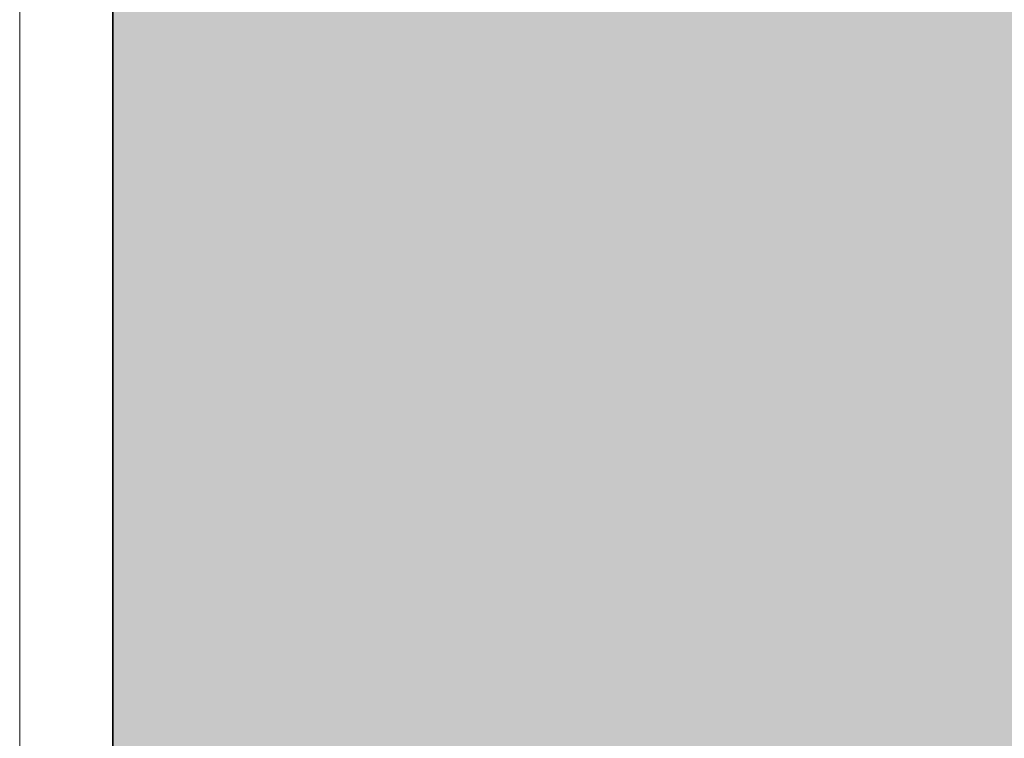
# Model space of a CAD drawing. Units: inches. Extents: x 2091 to 2899, y 967 to 2217.
# Tile 221 of 256: x 2203.1157 to 2203.4104, y 1152.4622 to 1152.6774. Entities that reach past the tile are written whole.
import ezdxf

# ---------------------------------------------------------------- set-up
doc = ezdxf.new("R2010")
doc.units = ezdxf.units.IN
doc.layers.add('A-GLAZ', color=4, linetype='Continuous', lineweight=18)
doc.layers.add('C-PROP', color=7, linetype='Continuous', lineweight=35)
doc.layers.add('A-WALL-PATT', color=141, linetype='Continuous', lineweight=13, true_color=0xadddf7)

# ---------------------------------------------------------------- blocks, each defined once
blk = doc.blocks.new('WIN-DOUBLE-LINE')
blk.add_line((0.0004, -0.00045), (0.0004, 80.8229))

msp = doc.modelspace()

# ---------------------------------------------------------------- hatches: boundary and pattern name
at = {"layer": 'A-WALL-PATT'}
h = msp.add_hatch(color=256, dxfattribs=at)
h.dxf.hatch_style = 1
h.paths.add_polyline_path([(2803.1436, 2050.91906), (2203.1436, 2050.91906), (2203.1436, 1090.91906), (2803.1436, 1090.91906)])
h.paths.add_polyline_path([(2635.79885, 1147.54046), (2674.52405, 1147.54046, 0.376086), (2678.52967, 1152.8802), (2678.52967, 1159.55647, 0.333335), (2674.52432, 1163.56185), (2674.52432, 1163.56185), (2674.52432, 1192.93439), (2635.80597, 1192.93439), (2597.08762, 1192.93439), (2597.08762, 1163.56185, 0.333335), (2593.08228, 1159.55647), (2593.08228, 1152.8802, 0.376086), (2597.08789, 1147.54046)], flags=0)
h.paths.add_polyline_path([(2436.01043, 1278.24078, 0.000483), (2435.95264, 1278.21503, -0.001328), (2435.93563, 1278.11169, -0.001711), (2436.11644, 1278.04076, 0.002185)], flags=0)
h.paths.add_polyline_path([(2794.1436, 1143.41906), (2794.1436, 1347.41906), (2543.37017, 1347.41906), (2543.37017, 1351.91906), (2794.1436, 1351.91906), (2794.1436, 1392.71355), (2793.9474, 1392.71355), (2793.9474, 1473.5369), (2794.1436, 1473.5369), (2794.1436, 1531.91906), (2650.1436, 1531.91906), (2650.1436, 1536.41906), (2794.1436, 1536.41906), (2794.1436, 1692.41906), (2609.37561, 1692.41906), (2609.37561, 1644.41906), (2604.87561, 1644.41906), (2604.87561, 1744.91906), (2609.37561, 1744.91906), (2609.37561, 1696.91906), (2794.1436, 1696.91906), (2794.1436, 1780.91906), (2609.6436, 1780.91906), (2493.87561, 1780.91906), (2493.87561, 1785.41906), (2609.6436, 1785.41906), (2794.1436, 1785.41906), (2794.1436, 1847.93882), (2793.95122, 1847.93882), (2793.95122, 1928.76217), (2794.1436, 1928.76217), (2794.1436, 1941.41906), (2614.1436, 1941.41906), (2614.1436, 1821.41906), (2609.6436, 1821.41906), (2609.6436, 1941.41906), (2392.1436, 1941.41906), (2392.1436, 1819.91906), (2387.6436, 1819.91906), (2387.6436, 1941.41906), (2212.1436, 1941.41906), (2212.1436, 1783.91906), (2392.1436, 1783.91906), (2392.1436, 1780.91906), (2212.1436, 1780.91906), (2212.1436, 1629.41906), (2387.6436, 1629.41906), (2387.6436, 1744.91906), (2392.1436, 1744.91906), (2392.1436, 1627.91906), (2317.1436, 1627.91906), (2317.1436, 1551.41906), (2317.1436, 1536.41906), (2459.38359, 1536.41906), (2459.38359, 1602.39648), (2463.88359, 1602.39648), (2463.88359, 1531.91906), (2456.6436, 1531.91906), (2456.6436, 1529.91906), (2452.1436, 1529.91906), (2452.1436, 1531.91906), (2312.6436, 1531.91906), (2312.6436, 1551.41906), (2306.1436, 1551.41906), (2306.1436, 1555.91906), (2308.1436, 1555.91906), (2308.1436, 1551.41906), (2312.6436, 1551.41906), (2312.6436, 1627.91906), (2212.1436, 1627.91906), (2212.1436, 1555.91906), (2270.1436, 1555.91906), (2270.1436, 1551.41906), (2212.1436, 1551.41906), (2212.1436, 1351.91906), (2272.1436, 1351.91906), (2272.1436, 1347.41906), (2212.1436, 1347.41906), (2212.1436, 1275.41906), (2308.1436, 1275.41906), (2308.1436, 1351.91906), (2452.1436, 1351.91906), (2452.1436, 1493.91906), (2456.6436, 1493.91906), (2456.6436, 1347.41906), (2312.6436, 1347.41906), (2312.6436, 1270.91906), (2212.1436, 1270.91906), (2212.1436, 1099.91906), (2281.23752, 1099.91906), (2282.87104, 1110.9138), (2282.00834, 1116.9966), (2278.55774, 1121.4204), (2268.20564, 1128.0562), (2272.08764, 1128.0562), (2273.81294, 1131.927), (2279.42034, 1134.6919), (2285.02784, 1135.2449), (2287.61584, 1137.4568), (2288.04714, 1138.0098), (2289.34114, 1140.7747), (2291.06654, 1139.6687), (2292.36054, 1135.2449), (2295.37984, 1136.9038), (2296.24254, 1135.7979), (2297.10524, 1133.033), (2300.12464, 1138.0098), (2303.14394, 1138.0098), (2304.43794, 1135.7979), (2303.14394, 1133.586), (2306.59464, 1134.6919), (2307.88874, 1133.033), (2310.90804, 1135.2449), (2313.92744, 1134.1389), (2315.62686, 1132.4271), (2308.32004, 1117.5496), (2290.20384, 1109.8079), (2288.90984, 1103.1721), (2289.27231, 1099.91906), (2434.91823, 1099.91906), (2431.59323, 1124.78806), (2429.93023, 1169.55306), (2430.92718, 1240.51969), (2435.65893, 1238.18613), (2437.13523, 1196.55406), (2438.79823, 1143.97306), (2442.67823, 1111.99806), (2446.55823, 1099.91906), (2794.1436, 1099.91906), (2794.1436, 1138.91906), (2548.03245, 1138.91906), (2548.03245, 1143.41906), (2548.03245, 1148.81906), (2546.66846, 1148.03156), (2528.68569, 1179.17862, 0.256256), (2512.03245, 1148.81906), (2512.03245, 1143.41906), (2512.03245, 1138.91906), (2507.53245, 1138.91906), (2507.53245, 1143.41906), (2507.53245, 1148.81906, 0.256256), (2490.8792, 1179.17862), (2472.89644, 1148.03156), (2471.53245, 1148.81906), (2471.53245, 1143.41906), (2467.03245, 1143.41906), (2467.03245, 1269.94579, 0.039061), (2460.90999, 1273.58006), (2467.03245, 1273.58006), (2467.03245, 1286.32536, 0.014511), (2465.21619, 1286.76191), (2467.03245, 1287.05258), (2467.03245, 1323.41906), (2471.53245, 1323.41906), (2471.53245, 1148.81906), (2489.53245, 1179.99597), (2490.89644, 1179.20847), (2490.8792, 1179.17862, -0.256256), (2507.53245, 1148.81906), (2507.53245, 1143.41906), (2512.03245, 1143.41906), (2512.03245, 1148.81906, -0.256256), (2528.68569, 1179.17862), (2528.66846, 1179.20847), (2530.03245, 1179.99597), (2548.03245, 1148.81906), (2548.03245, 1143.41906)], flags=16)
h.paths.add_polyline_path([(2607.76855, 1200.94508), (2607.76855, 1265.03063), (2597.08762, 1281.05201), (2619.78459, 1281.05201), (2627.79528, 1337.12686), (2635.79885, 1337.12686), (2643.81666, 1337.12686), (2651.82736, 1281.05201), (2674.52432, 1281.05201), (2663.8434, 1265.03063), (2663.8434, 1200.94508), (2635.80597, 1200.94508)], flags=0)
edge = h.paths.add_edge_path(flags=0)
edge.add_ellipse((13303.89622, 1272.99872), major_axis=(-10595.31304, 0), ratio=0.84230387009, start_angle=0.628237219, end_angle=0.6465541, ccw=False)
edge.add_ellipse((2711.70045, 1156.85268), major_axis=(2.21977, 0), ratio=0.8423039, start_angle=111.53524, end_angle=180.62824, ccw=False)
edge.add_ellipse((13303.15629, 1272.99872), major_axis=(-10593.02631, 0), ratio=0.84230386954, start_angle=0.528271472, end_angle=0.646554097, ccw=False)
edge.add_line((2710.7646, 1175.3333), (2710.12999, 1175.3333))
edge.add_ellipse((2710.12999, 1176.57978), major_axis=(1.47985, 0), ratio=0.8423039, start_angle=180, end_angle=270, ccw=False)
edge.add_line((2708.65014, 1176.57978), (2708.65014, 1200.78291))
edge.add_ellipse((2710.12999, 1200.78291), major_axis=(1.47985, 0), ratio=0.8423039, start_angle=90, end_angle=180, ccw=False)
edge.add_line((2710.12999, 1202.02939), (2710.46508, 1202.02939))
edge.add_ellipse((13303.15629, 1272.99872), major_axis=(-10593.02631, 0), ratio=0.84230386954, start_angle=-0.090229089, end_angle=0.383866779, ccw=False)
edge.add_ellipse((2710.12999, 1290.92703), major_axis=(-1.47985, 0), ratio=0.8423039, start_angle=0, end_angle=90, ccw=False)
edge.add_line((2708.65014, 1290.92703), (2708.65014, 1315.13017))
edge.add_ellipse((2710.12999, 1315.13017), major_axis=(-1.47985, 0), ratio=0.8423039, start_angle=-90, end_angle=0, ccw=False)
edge.add_line((2710.12999, 1316.37665), (2710.70631, 1316.37665))
edge.add_ellipse((3238.40172, 1296.28957), major_axis=(528.234, 0), ratio=0.84230387, start_angle=176.3495724, end_angle=177.8200497, ccw=False)
edge.add_ellipse((2775.06304, 1071.4507), major_axis=(313.30776, 0), ratio=0.84230387, start_angle=102.1259656, end_angle=103.780529, ccw=False)
edge.add_ellipse((2775.06304, 1078.3057), major_axis=(-305.30289, 0), ratio=0.84230387, start_angle=-79.790461, end_angle=-77.5553727, ccw=False)
edge.add_ellipse((2695.14177, 1541.97538), major_axis=(-250.96022, 0), ratio=0.84230387, start_angle=99.256566, end_angle=102.5549326)
edge.add_line((2741.41033, 1334.21426), (2747.13255, 1337.37848))
edge.add_ellipse((2747.53862, 1336.85748), major_axis=(-0.73992, 0), ratio=0.842304, start_angle=270, end_angle=307.93313, ccw=False)
edge.add_ellipse((2747.53862, 1336.85748), major_axis=(-0.73992, 0), ratio=0.842304, start_angle=232.06687, end_angle=270, ccw=False)
edge.add_line((2747.94469, 1337.37848), (2753.66691, 1334.21426))
edge.add_ellipse((2799.93547, 1541.97538), major_axis=(250.96022, 0), ratio=0.84230387, start_angle=257.4450674, end_angle=260.743434)
edge.add_ellipse((2720.01419, 1078.3057), major_axis=(305.30289, 0), ratio=0.84230387, start_angle=77.5553727, end_angle=79.790461, ccw=False)
edge.add_ellipse((2720.01419, 1071.4507), major_axis=(-313.30776, 0), ratio=0.84230387, start_angle=256.219471, end_angle=257.8740344, ccw=False)
edge.add_ellipse((2256.67551, 1296.28957), major_axis=(-528.234, 0), ratio=0.84230387, start_angle=182.1799503, end_angle=183.6504276, ccw=False)
edge.add_line((2784.37092, 1316.37665), (2784.94725, 1316.37665))
edge.add_ellipse((2784.94725, 1315.13017), major_axis=(1.47985, 0), ratio=0.8423039, start_angle=0, end_angle=90, ccw=False)
edge.add_line((2786.42709, 1315.13017), (2786.42709, 1290.92703))
edge.add_ellipse((2784.94725, 1290.92703), major_axis=(1.47985, 0), ratio=0.8423039, start_angle=270, end_angle=360, ccw=False)
edge.add_ellipse((-7808.07906, 1272.99872), major_axis=(10593.02631, 0), ratio=0.84230386954, start_angle=-0.383866779, end_angle=0.090229089, ccw=False)
edge.add_line((2784.61216, 1202.02939), (2784.94725, 1202.02939))
edge.add_ellipse((2784.94725, 1200.78291), major_axis=(1.47985, 0), ratio=0.8423039, start_angle=0, end_angle=90, ccw=False)
edge.add_line((2786.42709, 1200.78291), (2786.42709, 1176.57978))
edge.add_ellipse((2784.94725, 1176.57978), major_axis=(-1.47985, 0), ratio=0.8423039, start_angle=90, end_angle=180, ccw=False)
edge.add_line((2784.94725, 1175.3333), (2784.31264, 1175.3333))
edge.add_ellipse((-7808.07906, 1272.99872), major_axis=(10593.02631, 0), ratio=0.84230386954, start_angle=-0.618643196, end_angle=-0.528271472, ccw=False)
edge.add_ellipse((2783.37678, 1156.85268), major_axis=(-2.21977, 0), ratio=0.8423039, start_angle=179.37176, end_angle=248.46476, ccw=False)
edge.add_ellipse((-7808.81898, 1272.99872), major_axis=(-10595.31304, 0), ratio=0.84230386576, start_angle=179.353445923, end_angle=179.371762803, ccw=False)
edge.add_ellipse((2780.2973, 1153.50079), major_axis=(-5.24643, 0), ratio=0.8423039, start_angle=90, end_angle=179.35345, ccw=False)
edge.add_line((2780.2973, 1149.08171), (2714.77993, 1149.08171))
edge.add_ellipse((2714.77993, 1153.50079), major_axis=(5.24643, 0), ratio=0.8423039, start_angle=180.64655, end_angle=270, ccw=False)
edge = h.paths.add_edge_path(flags=0)
edge.add_line((2718.18737, 1151.00783), (2718.18737, 1170.47236))
edge.add_ellipse((2721.14706, 1170.47236), major_axis=(-2.95969, 0), ratio=0.8423039, start_angle=-90, end_angle=0, ccw=False)
edge.add_line((2721.14706, 1172.96532), (2773.93017, 1172.96532))
edge.add_ellipse((2773.93017, 1170.47236), major_axis=(-2.95969, 0), ratio=0.8423039, start_angle=180, end_angle=270, ccw=False)
edge.add_line((2776.88987, 1170.47236), (2776.88987, 1151.00783))
edge.add_line((2776.88987, 1151.00783), (2718.18737, 1151.00783))
edge = h.paths.add_edge_path(flags=0)
edge.add_line((2718.18737, 1180.23415), (2718.18737, 1199.05783))
edge.add_ellipse((2747.53862, 1320.39864), major_axis=(147.01792, 0), ratio=0.84230387, start_angle=256.4018653, end_angle=283.5981347)
edge.add_line((2776.88987, 1199.05783), (2776.88987, 1180.23415))
edge.add_ellipse((2747.53862, 1301.57496), major_axis=(147.01792, 0), ratio=0.84230387, start_angle=256.4018653, end_angle=283.5981347, ccw=False)
edge = h.paths.add_edge_path(flags=0)
edge.add_ellipse((13303.15629, 1272.99872), major_axis=(-10591.54646, 0), ratio=0.84230386955, start_angle=0.055594314, end_angle=0.377764194, ccw=False)
edge.add_line((2711.61686, 1262.72171), (2715.66741, 1249.4954))
edge.add_ellipse((6413.89196, 1241.69192), major_axis=(-3698.23616, 0), ratio=0.8423038695, start_angle=-0.12089737, end_angle=0.36407635)
edge.add_line((2715.76104, 1218.19245), (2711.93431, 1203.16736))
edge = h.paths.add_edge_path(flags=0)
edge.add_line((2718.18737, 1251.07457), (2716.00249, 1267.45044))
edge.add_ellipse((2742.15117, 1202.18954), major_axis=(81.77258, 0), ratio=0.84230387, start_angle=94.277421, end_angle=111.8349538, ccw=False)
edge.add_line((2737.00975, 1270.93063), (2758.06748, 1270.93063))
edge.add_ellipse((2752.92606, 1202.18954), major_axis=(81.77258, 0), ratio=0.84230387, start_angle=68.1650462, end_angle=85.722579, ccw=False)
edge.add_line((2779.07475, 1267.45044), (2776.88987, 1251.07457))
edge.add_ellipse((2750.33806, 1187.88536), major_axis=(79.57966, 0), ratio=0.84230387, start_angle=67.2080851, end_angle=85.1299304)
edge.add_line((2756.03466, 1254.74366), (2739.04258, 1254.74366))
edge.add_ellipse((2744.73917, 1187.88536), major_axis=(79.57966, 0), ratio=0.84230387, start_angle=94.8700696, end_angle=112.7919149)
edge = h.paths.add_edge_path(flags=0)
edge.add_line((2783.14293, 1203.16736), (2779.31619, 1218.19245))
edge.add_ellipse((-918.81473, 1241.69192), major_axis=(3698.23616, 0), ratio=0.8423038695, start_angle=-0.36407635, end_angle=0.12089737)
edge.add_line((2779.40983, 1249.4954), (2783.46037, 1262.72171))
edge.add_ellipse((-7808.07906, 1272.99872), major_axis=(-10591.54646, 0), ratio=0.84230386954, start_angle=179.622235806, end_angle=179.944405687, ccw=False)
edge = h.paths.add_edge_path(flags=0)
edge.add_ellipse((2734.20089, 1286.69044), major_axis=(-0.35661, 6.34008), ratio=0.6038336, start_angle=89.002014, end_angle=253.657408, ccw=False)
edge.add_line((2730.369, 1286.54181), (2730.369, 1301.35198))
edge.add_line((2730.369, 1301.35198), (2735.91331, 1305.2148))
edge.add_ellipse((2736.38492, 1304.73456), major_axis=(0.73992, 0), ratio=0.842304, start_angle=90, end_angle=134.48021, ccw=False)
edge.add_line((2736.38492, 1305.3578), (2738.03278, 1305.3578))
edge.add_line((2738.03278, 1305.3578), (2738.03278, 1307.70793))
edge.add_ellipse((2794.20164, 1307.70793), major_axis=(56.16886, 0), ratio=0.84230387, start_angle=150.56143, end_angle=180, ccw=False)
edge.add_ellipse((2700.87559, 1307.70793), major_axis=(-56.16886, 0), ratio=0.84230387, start_angle=180, end_angle=209.43857, ccw=False)
edge.add_line((2757.04445, 1307.70793), (2757.04445, 1305.3578))
edge.add_line((2757.04445, 1305.3578), (2758.69232, 1305.3578))
edge.add_ellipse((2758.69232, 1304.73456), major_axis=(-0.73992, 0), ratio=0.842304, start_angle=225.51979, end_angle=270, ccw=False)
edge.add_line((2759.16392, 1305.2148), (2764.70823, 1301.35198))
edge.add_line((2764.70823, 1301.35198), (2764.70823, 1286.54181))
edge.add_ellipse((2760.87634, 1286.69044), major_axis=(0.35661, 6.34008), ratio=0.6038336, start_angle=106.342592, end_angle=270.997986, ccw=False)
edge.add_line((2757.04445, 1285.79709), (2757.04445, 1307.70793))
edge.add_ellipse((2700.87559, 1307.70793), major_axis=(-56.16886, 0), ratio=0.84230387, start_angle=180, end_angle=209.43857)
edge.add_ellipse((2794.20164, 1307.70793), major_axis=(56.16886, 0), ratio=0.84230387, start_angle=150.56143, end_angle=180)
edge.add_line((2738.03278, 1307.70793), (2738.03278, 1285.79709))
h.paths.add_polyline_path([(2417.81227, 1104.4497), (2413.49227, 1102.5297), (2410.61227, 1103.9697), (2409.17227, 1106.3697), (2407.25227, 1107.3297), (2406.29227, 1109.7297), (2405.33227, 1114.0497), (2405.33227, 1117.8897), (2406.29227, 1120.1297), (2407.25227, 1119.8097), (2408.84832, 1118.32766), (2410.17395, 1119.42417), (2410.21127, 1120.4057), (2411.04073, 1121.41905), (2410.69927, 1119.8587), (2410.17395, 1119.42417), (2410.08845, 1117.17611), (2411.13284, 1116.20632), (2413.97227, 1119.3297), (2416.85227, 1120.7697), (2416.86972, 1120.79878), (2417.03507, 1119.40512), (2417.89621, 1118.14338), (2418.29227, 1118.3697), (2419.54445, 1120.03927), (2419.36092, 1118.38749), (2419.03211, 1119.35615), (2418.39894, 1118.51193), (2419.25227, 1114.5297), (2418.79409, 1107.19879)], flags=0)
h.paths.add_polyline_path([(2508.87017, 1347.41906), (2508.37017, 1347.41906), (2508.37017, 1351.91906), (2508.87017, 1351.91906)], flags=0)
h.paths.add_polyline_path([(2473.37017, 1347.41906), (2472.37017, 1347.41906), (2467.87017, 1347.41906), (2467.87017, 1455.41906), (2472.37017, 1455.41906), (2472.37017, 1352.41906), (2473.37017, 1352.41906)], flags=0)
h.paths.add_polyline_path([(2352.10624, 1217.4462), (2349.22624, 1218.8862), (2347.78624, 1221.2862), (2345.86624, 1222.2462), (2344.90624, 1224.6462), (2343.94624, 1228.9662), (2343.94624, 1232.8062), (2344.90624, 1235.0462), (2345.86624, 1234.7262), (2347.46229, 1233.24415), (2348.78792, 1234.34066), (2348.82524, 1235.3222), (2349.6547, 1236.33555), (2349.31324, 1234.7752), (2348.78792, 1234.34066), (2348.70242, 1232.0926), (2349.74681, 1231.12282), (2352.58624, 1234.2462), (2355.46624, 1235.6862), (2355.48369, 1235.71528), (2355.64904, 1234.32161), (2356.51018, 1233.05988), (2356.90624, 1233.2862), (2358.15842, 1234.95576), (2357.97489, 1233.30398), (2357.64608, 1234.27264), (2357.01291, 1233.42842), (2357.86624, 1229.4462), (2357.40806, 1222.11529), (2356.42624, 1219.3662)], flags=0)
h.paths.add_polyline_path([(2348.2968, 1112.22442), (2347.0138, 1112.31042), (2345.5298, 1114.12742), (2345.7318, 1115.85842), (2346.8118, 1116.98242), (2346.8118, 1114.64642), (2345.8668, 1114.21442), (2346.8798, 1114.30042)], flags=0)
h.paths.add_polyline_path([(2347.0138, 1110.92642), (2346.2718, 1110.49342), (2346.6098, 1111.18642)], flags=0)
h.paths.add_polyline_path([(2345.8668, 1118.19442), (2345.5298, 1117.32942), (2343.7078, 1118.02142), (2344.3828, 1118.62642)], flags=0)
h.paths.add_polyline_path([(2346.6768, 1109.28242), (2346.0698, 1108.07142), (2345.8668, 1110.06142)], flags=0)
h.paths.add_polyline_path([(2345.0568, 1119.75142), (2343.6398, 1119.75142), (2343.9778, 1121.13542)], flags=0)
h.paths.add_polyline_path([(2345.2598, 1116.55042), (2345.1248, 1115.85842), (2344.9218, 1115.68542), (2344.7198, 1116.37742)], flags=0)
h.paths.add_polyline_path([(2345.6648, 1112.31042), (2345.4618, 1111.53242), (2344.0448, 1111.96442), (2344.6518, 1112.57042)], flags=0)
h.paths.add_polyline_path([(2345.1918, 1113.34942), (2344.4498, 1113.86842), (2344.7198, 1114.38742)], flags=0)
h.paths.add_polyline_path([(2344.6518, 1116.80942), (2344.1798, 1115.68542), (2344.6518, 1115.33942), (2343.9098, 1114.90642), (2343.0328, 1115.94442), (2343.6398, 1116.46342)], flags=0)
h.paths.add_polyline_path([(2345.8668, 1106.68642), (2344.9898, 1105.56242), (2344.5168, 1106.60042)], flags=0)
h.paths.add_polyline_path([(2344.8548, 1110.06142), (2344.5168, 1109.28242), (2344.1128, 1109.71542)], flags=0)
h.paths.add_polyline_path([(2344.0448, 1113.52242), (2343.4378, 1113.08942), (2342.7628, 1113.95442)], flags=0)
h.paths.add_polyline_path([(2344.3148, 1111.01242), (2342.9648, 1110.32042), (2342.9648, 1111.09942)], flags=0)
h.paths.add_polyline_path([(2345.1248, 1104.69742), (2344.5848, 1103.74542), (2344.4498, 1104.26442)], flags=0)
h.paths.add_polyline_path([(2342.8298, 1121.22242), (2341.7498, 1120.53042), (2340.5358, 1121.04942), (2340.1308, 1121.82842), (2340.6708, 1122.95242), (2341.1428, 1121.82842), (2341.6148, 1122.00142)], flags=0)
h.paths.add_polyline_path([(2342.9648, 1119.75142), (2343.0328, 1118.45342), (2342.0878, 1118.02142), (2342.0198, 1119.49142)], flags=0)
h.paths.add_polyline_path([(2342.6948, 1116.89642), (2341.9528, 1116.63642), (2342.0198, 1117.32942)], flags=0)
h.paths.add_polyline_path([(2343.0328, 1112.22442), (2342.0198, 1111.79142), (2341.5478, 1112.22442), (2342.3578, 1113.34942)], flags=0)
h.paths.add_polyline_path([(2343.7748, 1104.43742), (2342.6278, 1102.88042), (2342.6948, 1104.61042), (2343.4378, 1105.12942)], flags=0)
h.paths.add_polyline_path([(2342.0198, 1115.07942), (2340.8058, 1115.51242), (2340.9408, 1116.37742)], flags=0)
h.paths.add_polyline_path([(2341.4808, 1120.09742), (2341.4808, 1119.40542), (2341.0758, 1119.57842), (2341.1428, 1120.09742)], flags=0)
h.paths.add_polyline_path([(2341.8178, 1114.47342), (2340.9408, 1113.08942), (2340.8058, 1114.56042)], flags=0)
h.paths.add_polyline_path([(2341.1428, 1118.54042), (2340.9408, 1116.98242), (2339.0508, 1117.67542), (2339.0508, 1118.62642)], flags=0)
h.paths.add_polyline_path([(2342.6948, 1101.66842), (2341.9528, 1101.84142), (2342.5598, 1102.36142)], flags=0)
h.paths.add_polyline_path([(2340.3328, 1119.66542), (2338.4438, 1119.57842), (2337.9038, 1120.35742), (2339.6578, 1120.61642)], flags=0)
h.paths.add_polyline_path([(2340.3328, 1115.33942), (2340.0628, 1113.69542), (2339.3878, 1115.33942)], flags=0)
h.paths.add_polyline_path([(2341.8178, 1103.83142), (2341.5478, 1102.88042), (2341.1428, 1103.65842)], flags=0)
h.paths.add_polyline_path([(2339.0508, 1122.86642), (2337.2958, 1121.82842), (2337.0938, 1123.12542), (2337.7688, 1123.81842)], flags=0)
h.paths.add_polyline_path([(2339.1178, 1121.74142), (2338.8478, 1121.22242), (2338.1738, 1121.04942), (2338.3758, 1121.56842)], flags=0)
h.paths.add_polyline_path([(2339.1858, 1119.31942), (2338.6458, 1118.71342), (2338.2408, 1118.10742), (2338.2408, 1118.88642)], flags=0)
h.paths.add_polyline_path([(2341.1428, 1101.92842), (2340.6028, 1101.23642), (2340.0628, 1101.84142), (2340.6028, 1102.36142)], flags=0)
h.paths.add_polyline_path([(2337.6338, 1117.76142), (2336.6208, 1118.28042), (2337.2958, 1118.97242)], flags=0)
h.paths.add_polyline_path([(2336.8238, 1119.57842), (2334.7988, 1118.97242), (2335.2038, 1120.35742), (2336.5538, 1120.87642)], flags=0)
h.paths.add_polyline_path([(2339.1178, 1100.45742), (2337.3638, 1100.54342), (2336.7558, 1101.23642)], flags=0)
h.paths.add_polyline_path([(2336.3508, 1122.43342), (2336.0138, 1121.91442), (2334.9338, 1122.43342), (2334.5288, 1123.47142), (2335.7438, 1122.77942)], flags=0)
h.paths.add_polyline_path([(2334.7318, 1120.87642), (2334.2588, 1120.35742), (2334.0568, 1120.78942), (2334.5968, 1121.30842)], flags=0)
h.paths.add_polyline_path([(2334.4618, 1122.17442), (2332.5718, 1121.30842), (2331.3568, 1122.17442), (2332.0998, 1122.86642)], flags=0)
h.paths.add_polyline_path([(2334.2588, 1118.54042), (2333.3818, 1118.45342), (2333.6518, 1119.31942)], flags=0)
h.paths.add_polyline_path([(2335.5418, 1102.27442), (2334.1918, 1102.62042), (2335.2718, 1103.31242)], flags=0)
h.paths.add_polyline_path([(2332.7068, 1119.66542), (2331.6948, 1120.44342), (2332.5048, 1120.78942)], flags=0)
h.paths.add_polyline_path([(2334.7318, 1101.14942), (2333.5168, 1101.58242), (2333.9888, 1101.75542)], flags=0)
h.paths.add_polyline_path([(2332.6398, 1116.63642), (2331.0868, 1116.29042), (2331.9648, 1118.19442)], flags=0)
h.paths.add_polyline_path([(2330.7498, 1121.56842), (2330.2768, 1120.27042), (2328.5228, 1119.31942), (2328.9948, 1121.04942)], flags=0)
h.paths.add_polyline_path([(2330.7498, 1118.62642), (2330.0078, 1117.50242), (2329.8728, 1118.02142)], flags=0)
h.paths.add_polyline_path([(2332.0998, 1102.36142), (2330.5468, 1102.01442), (2331.6948, 1102.96642)], flags=0)
h.paths.add_polyline_path([(2329.5348, 1113.60842), (2329.0628, 1112.31042), (2328.5898, 1113.34942)], flags=0)
h.paths.add_polyline_path([(2328.3878, 1117.84842), (2327.5098, 1116.55042), (2327.1728, 1117.76142)], flags=0)
h.paths.add_polyline_path([(2329.7378, 1106.51342), (2329.5348, 1105.30242), (2328.2528, 1106.08142)], flags=0)
h.paths.add_polyline_path([(2328.6578, 1114.38742), (2328.0498, 1114.12742), (2328.3198, 1114.90642)], flags=0)
h.paths.add_polyline_path([(2328.3198, 1112.22442), (2327.1058, 1112.13742), (2326.7008, 1112.65642)], flags=0)
h.paths.add_polyline_path([(2326.9028, 1115.25242), (2326.7008, 1114.12742), (2325.2158, 1113.60842), (2326.0928, 1115.33942)], flags=0)
h.paths.add_polyline_path([(2326.6328, 1108.33042), (2326.0928, 1107.37942), (2325.8908, 1108.50342), (2326.4978, 1109.10942)], flags=0)
h.paths.add_polyline_path([(2615.1436, 1531.91906), (2609.6436, 1531.91906), (2609.6436, 1620.41906), (2614.1436, 1620.41906), (2614.1436, 1536.41906), (2615.1436, 1536.41906)], flags=0)
h.paths.add_polyline_path([(2545.1436, 1563.41906), (2464.1436, 1563.41906), (2464.1436, 1632.41906), (2509.1436, 1632.41906), (2509.1436, 1627.91906), (2509.1436, 1603.91906), (2468.6436, 1603.91906), (2468.6436, 1567.91906), (2540.6436, 1567.91906), (2540.6436, 1591.91906), (2545.1436, 1591.91906)], flags=0)
h.paths.add_polyline_path([(2388.96905, 1549.98573), (2357.43418, 1549.98573), (2357.43418, 1623.36078), (2399.36278, 1623.36078), (2435.68947, 1623.36078), (2435.59255, 1602.55927), (2435.59255, 1602.39648), (2388.96905, 1602.39648)], flags=0)
h.paths.add_polyline_path([(2388.88063, 1555.80915), (2374.90443, 1555.80915), (2374.90443, 1600.57156), (2374.90443, 1615.45765), (2406.35088, 1615.45765), (2406.35088, 1618.93943), (2412.17429, 1615.45765), (2406.35088, 1611.97586), (2406.35088, 1615.45765), (2388.88063, 1615.45765)], flags=0)
h.paths.add_polyline_path([(2568.87561, 1644.41906), (2453.37561, 1644.41906), (2453.37561, 1785.41906), (2457.87561, 1785.41906), (2457.87561, 1648.91906), (2568.87561, 1648.91906)], flags=0)
h.paths.add_polyline_path([(2212.1436, 1945.91906), (2212.1436, 2041.91906), (2794.1436, 2041.91906), (2794.1436, 1945.91906)], flags=16)
h.paths.add_polyline_path([(2271.08273, 1964.31724), (2776.85297, 1964.31724), (2776.85297, 2037.16962), (2271.08273, 2037.16962)], flags=8)
h.paths.add_polyline_path([(2380.64929, 1536.82414), (2461.04081, 1536.82414), (2461.04081, 1554.65259), (2380.64929, 1554.65259)], flags=8)
h.paths.add_polyline_path([(2240.75571, 1609.72545), (2309.18583, 1609.72545), (2309.18583, 1617.6982), (2240.75571, 1617.6982)], flags=8)
h.paths.add_polyline_path([(2212.67726, 1313.5041), (2282.59152, 1313.5041), (2282.59152, 1322.74524), (2212.67726, 1322.74524)], flags=8)
h.paths.add_polyline_path([(2457.11198, 1114.77857), (2558.48158, 1114.77857), (2558.48158, 1142.21968), (2457.11198, 1142.21968)], flags=8)
h.paths.add_polyline_path([(2473.44234, 1273.01007), (2604.64123, 1273.01007), (2604.64123, 1318.34693), (2473.44234, 1318.34693)], flags=8)
h.paths.add_polyline_path([(2638.8763, 1626.97743), (2684.25037, 1627.97674), (2684.03848, 1637.59749), (2638.66442, 1636.59819)], flags=8)
h.paths.add_polyline_path([(2537.59055, 1453.79345), (2628.38955, 1453.79345), (2628.38955, 1475.34481), (2537.59055, 1475.34481)], flags=8)
h.paths.add_polyline_path([(2504.13764, 1714.6324), (2554.64719, 1714.6324), (2554.64719, 1730.23771), (2504.13764, 1730.23771)], flags=8)
h.paths.add_polyline_path([(2487.50118, 1575.65187), (2535.09712, 1575.65187), (2535.09712, 1598.37765), (2487.50118, 1598.37765)], flags=8)
h.paths.add_polyline_path([(2709.0994, 1735.71028), (2740.0166, 1735.71028), (2740.0166, 1749.93764), (2709.0994, 1749.93764)], flags=8)
h.paths.add_polyline_path([(2442.43842, 1792.17166), (2564.72884, 1792.17166), (2564.72884, 1842.00016), (2442.43842, 1842.00016)], flags=8)
h.paths.add_polyline_path([(2655.8158, 1809.64408), (2789.52014, 1806.6938), (2790.08498, 1832.29164), (2656.38064, 1835.24192)], flags=8)
h.paths.add_polyline_path([(2234.8427, 1797.72014), (2368.59285, 1794.76885), (2369.16072, 1820.50413), (2235.41056, 1823.45542)], flags=8)
h.paths.add_polyline_path([(2245.13847, 1644.00633), (2398.42773, 1640.6239), (2398.99484, 1666.32482), (2245.70557, 1669.70725)], flags=8)
h.paths.add_polyline_path([(2306.14285, 1431.16852), (2413.76831, 1428.79369), (2414.33315, 1454.39153), (2306.70768, 1456.76636)], flags=8)
h.paths.add_polyline_path([(2306.83458, 1458.23314), (2393.38048, 1456.32345), (2393.93281, 1481.35436), (2307.38691, 1483.26405)], flags=8)

# ---------------------------------------------------------------- linework, layer by layer
at = {"layer": 'C-PROP'}
msp.add_lwpolyline([(2203.1436, 2050.91906), (2803.1436, 2050.91906), (2803.1436, 1090.91906), (2203.1436, 1090.91906)], close=True, dxfattribs=at)

# ---------------------------------------------------------------- block references
at = {"layer": 'A-GLAZ'}
msp.add_blockref('WIN-DOUBLE-LINE', (2203.11534, 1152.2475), dxfattribs=at)

doc.saveas('drawing.dxf')
